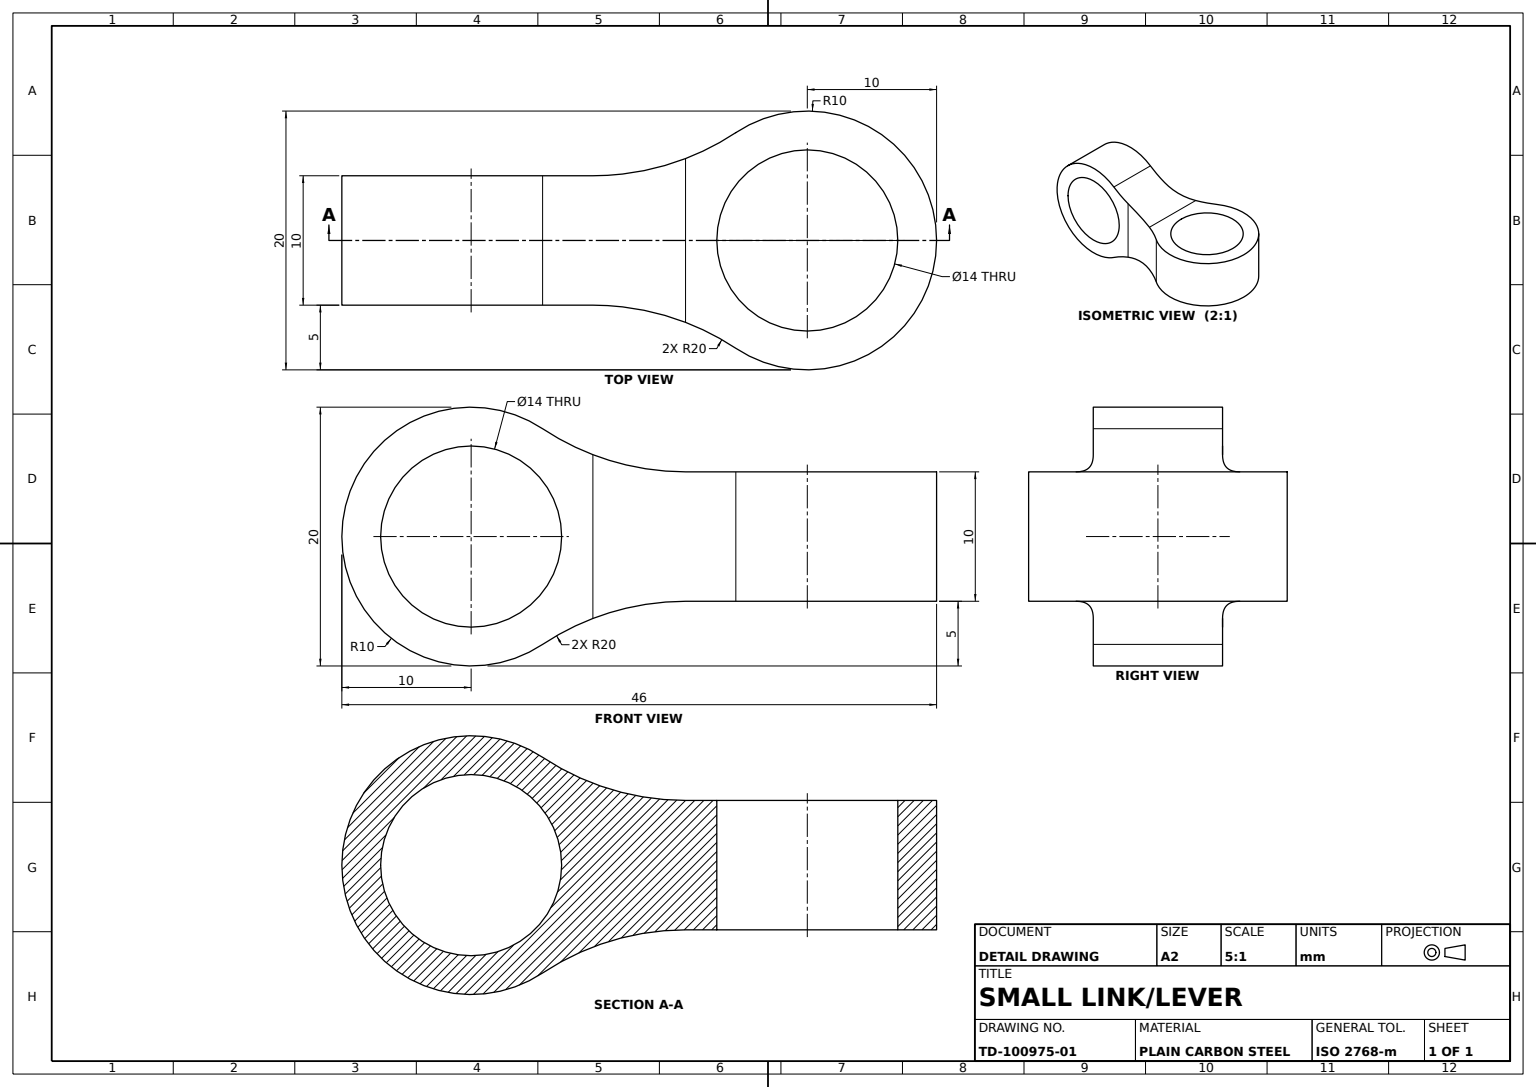
SolidWorks part; units mm, degrees
material "Plain Carbon Steel"
ref_plane "Front Plane" through (0, 0, 0) normal (0, 0, 1) x (1, 0, 0)
ref_plane "Top Plane" through (0, 0, 0) normal (0, 1, 0) x (1, 0, 0)
ref_plane "Right Plane" through (0, 0, 0) normal (1, 0, 0) x (0, 0, -1)
sketch "Link Block Sketch" plane through (0, 0, 0) normal (0, 0, 1) x (1, 0, 0)
  line L1 (-23, 10) -> (23, 10)
  line L2 (-23, 10) -> (-23, -10)
  line L3 (-23, -10) -> (23, -10)
  line L4 (23, 10) -> (23, -10)
  line L5 (-23, 10) -> (23, -10) construction
  line L6 (-23, -10) -> (23, 10) construction
  point P0 (0, 0)
  dimension "D1" = 20
  dimension "D2" = 46
extrude "Link Block" add sketch "Link Block Sketch" along normal mid plane 20
sketch "First Lug Profile Sketch" plane through (0, 0, 10) normal (0, 0, 1) x (1, 0, 0)
  line L0 (-23, 10) -> (-23, -10) construction
  line L1 (23, -10) -> (23, 10) construction
  line L2 (3.5831, 5) -> (23, 5)
  line L4 (3.5831, -5) -> (23, -5)
  line L6 (-22.0333, 5) -> (23, -5) construction
  line L7 (-22.0333, -5) -> (23, 5) construction
  line L12 (23, -10) -> (23, 10)
  line L13 (23, 10) -> (-23, 10)
  line L14 (-23, 10) -> (-23, -10)
  line L15 (-23, -10) -> (23, -10)
  line L16 (23, -10) -> (23, 10)
  line L17 (23, 10) -> (-23, 10)
  line L18 (-23, 10) -> (-23, -10)
  line L19 (-23, -10) -> (23, -10)
  arc A0 (-7.4723, 8.3333) -> (-7.4723, -8.3333) centre (-13, 0) ccw
  circle A1 centre (-13, 0) radius 7
  arc A2 (-7.4723, -8.3333) -> (3.5831, -5) centre (3.5831, -25) cw
  arc A3 (-7.4723, 8.3333) -> (3.5831, 5) centre (3.5831, 25) ccw
  point P9 (0.4833, 0)
  line M3 (23, -10) -> (23, 10)
  line M4 (23, 10) -> (-23, 10)
  line M5 (-23, 10) -> (-23, -10)
  line M6 (-23, -10) -> (23, -10)
  dimension "D1" = 20
  dimension "D4" = 14
  dimension "D5" = 20
  dimension "D2" = 10
  dimension "D3" = 5
  dimension "D7" = 22.0333
  dimension "D6" = 0
extrude "First Lug Profile & Bore Cut" cut sketch "First Lug Profile Sketch" against normal mid plane 70 contours A0 A3 L2 M3 M4 | A0 L17 M5 | A0 L18 M6 | A2 A0 L19 L4 M3 | A1
sketch "Second Lug Profile Sketch" plane through (0, -5, 0) normal (0, -1, 0) x (1, 0, 0)
  line L2 (-23, 5) -> (-3.5831, 5)
  line L3 (-23, 5) -> (-23, -5)
  line L4 (-23, -5) -> (-3.5831, -5)
  line L6 (3.5831, -10) -> (3.5831, 10) construction
  line L7 (-26.1665, 15.4159) -> (28.9555, 15.4159)
  line L8 (-26.1665, 15.4159) -> (-26.1665, -13.1339)
  line L9 (-26.1665, -13.1339) -> (28.9555, -13.1339)
  line L10 (28.9555, 15.4159) -> (28.9555, -13.1339)
  arc A0 (7.4723, -8.3333) -> (7.4723, 8.3333) centre (13, 0) ccw
  arc A1 (7.4723, -8.3333) -> (-3.5831, -5) centre (-3.5831, -25) ccw
  arc A2 (7.4723, 8.3333) -> (-3.5831, 5) centre (-3.5831, 25) cw
  circle A3 centre (13, 0) radius 7
  line M3 (3.5831, 10) -> (3.5831, -10)
  line M4 (3.5831, -10) -> (23, -10)
  line M5 (23, -10) -> (23, 10)
  line M6 (23, 10) -> (3.5831, 10)
  dimension "D1" = 20
  dimension "D4" = 20
  dimension "D5" = 14
  dimension "D2" = 10
  dimension "D3" = 5
  dimension "D6" = 3.8892
  dimension "D7" = 25.3724
  dimension "D8" = 26.5831
  dimension "D9" = 29.7496
  dimension "D10" = 5.4159
  dimension "D11" = 23.1339
extrude "Second Lug Profile & Bore Cut" cut sketch "Second Lug Profile Sketch" against normal mid plane 70 contours L10 L7 L8 L9 A2 A1 L4 L3 L2 M3 M6 M5 M4 | A3 | A0 M4 M5 | A0 A1 M3 M4 | A2 A0 M6 M3 | A0 M5 M6
